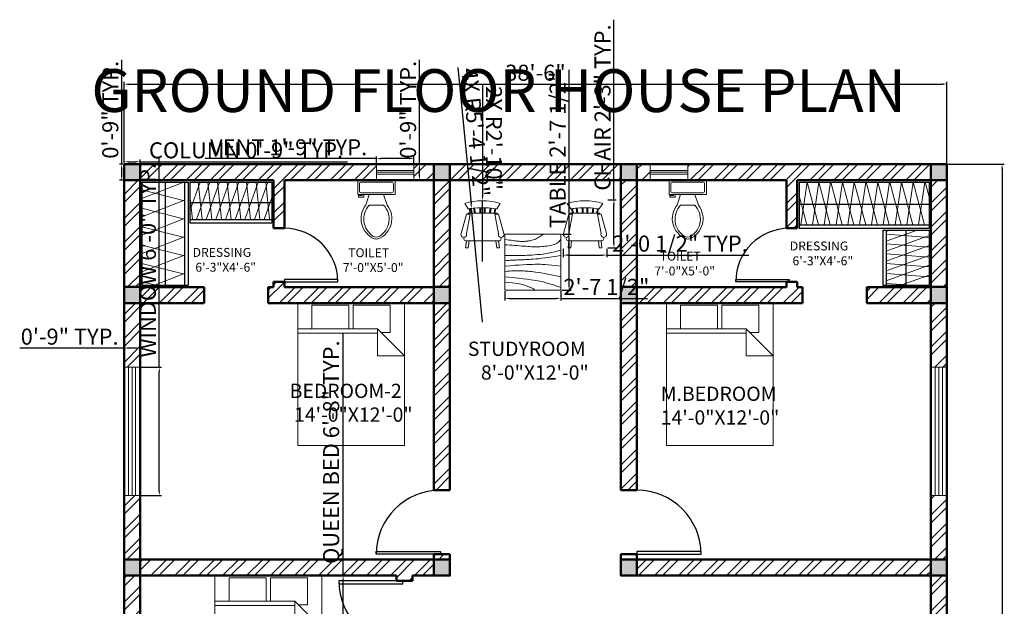
# Model space of a CAD drawing. Units: inches. Extents: x 381 to 1001, y 3003 to 3971.
# Tile 4 of 4: x 419 to 972, y 3641 to 3971. Entities that reach past the tile are written whole.
import ezdxf

# ---------------------------------------------------------------- set-up
doc = ezdxf.new("R2010")
doc.units = ezdxf.units.IN
for name, color, linetype, lineweight in [('A-ANNO-DIMS', 2, 'Continuous', 18), ('A-ANNO-TEXT', 7, 'Continuous', 25), ('A-AREA-IDEN', 7, 'Continuous', 18), ('A-COLS', 7, 'Continuous', 50), ('A-DOOR', 4, 'Continuous', 25), ('A-FLOR-CASE', 8, 'Continuous', 25), ('A-FLOR-CASE-PATT', 252, 'Continuous', 13), ('A-FLOR-FIXT', 9, 'Continuous', 18), ('A-FURN', 8, 'Continuous', 18), ('A-GLAZ', 244, 'Continuous', 18), ('A-WALL', 7, 'Continuous', 50), ('A-WALL-PATT', 252, 'Continuous', 13)]:
    doc.layers.add(name, color=color, linetype=linetype, lineweight=lineweight)
doc.styles.get("Standard").update_dxf_attribs({"font": 'arial.ttf'})
doc.dimstyles.new('ISO-25', dxfattribs={"dimtxt": 9, "dimasz": 2.5, "dimexe": 1.25, "dimexo": 0.625, "dimtad": 1, "dimlunit": 3, "dimtxsty": 'Standard', "dimcen": 2.5, "dimadec": 0, "dimazin": 0, "dimtfac": 1, "dimtmove": 0, "dimatfit": 3, "dimfxl": 1, "dimarcsym": 0})

# ---------------------------------------------------------------- blocks, each defined once
blk = doc.blocks.new('*U5')
for p, q in [((0, 0), (0, 6)), ((40, 0), (40, 6))]:
    blk.add_line(p, q)
blk.add_lwpolyline([(0, 0), (0, -40), (1.75, -40), (1.75, 0)], close=True)
blk.add_arc((0, 0), 40, 270, 360)
blk = doc.blocks.new('*U4')
for p, q in [((0, 0), (0, -6)), ((40, 0), (40, -6))]:
    blk.add_line(p, q)
blk.add_lwpolyline([(0, 0), (0, 40), (1.75, 40), (1.75, 0)], close=True)
blk.add_arc((0, 0), 40, 0, 90)
blk = doc.blocks.new('*U3')
for p, q in [((0, 0), (0, -6)), ((-40, 0), (-40, -6))]:
    blk.add_line(p, q)
blk.add_lwpolyline([(0, 0), (0, 40), (-1.75, 40), (-1.75, 0)], close=True)
blk.add_arc((0, 0), 40, 90, 180)
blk = doc.blocks.new('*U9')
for p, q in [((9.5, -6), (9.5, -2)), ((-10, -8.5), (-8, -8.5)), ((-10, -9.5), (-10, -8.5)), ((-7, -9.5), (-10, -9.5)), ((-8, -8.5), (-8, -8)), ((-7, -8), (-7, -9.5)), ((-4, -8), (-6, -14)), ((4, -8), (6, -14)), ((4, -14), (-4, -14))]:
    blk.add_line(p, q)
blk.add_lwpolyline([(10.5, -8), (10.5, 0), (-10.5, 0), (-10.5, -8)], close=True)
for points in [[(-9.5, -2), (-9.5, -6)], [(8.5, -1), (-8.5, -1)], [(-8.5, -7), (8.5, -7)]]:
    blk.add_lwpolyline(points)
for centre, radius, start, end in [((-8.62, -1.88), 0.884, 81.8699, 188.1301), ((8.62, -1.88), 0.884, 351.8699, 98.1301), ((-8.62, -6.12), 0.884, 171.8699, 278.1301), ((8.62, -6.12), 0.884, 261.8699, 8.1301), ((3.52, -21.58), 12.17, 141.4691, 247.9714), ((4.2, -21.82), 11.33, 136.3677, 238.9468), ((-3.52, -21.58), 12.17, 292.0284, 38.5307), ((-4.2, -21.82), 11.33, 301.053, 43.6321), ((0, -27.88), 4, 245.7318, 294.2682), ((0, -29), 4, 254.8605, 285.1395)]:
    blk.add_arc(centre, radius, start, end)
blk = doc.blocks.new('Bed - Queen')
for p, q in [((0, -80.00003), (0, 0)), ((0, 0), (59.99999, 0)), ((59.99999, 0), (59.99999, -80.00003)), ((7.99999, -1.2), (28.79998, -1.2)), ((7.99999, -14.4), (7.99999, -1.2)), ((28.79998, -1.2), (28.79998, -14.4)), ((31.19999, -1.2), (51.99999, -1.2)), ((31.19999, -14.4), (31.19999, -1.2)), ((51.99999, -1.2), (51.99999, -16.4)), ((0, -14.4), (44.8, -14.4)), ((59.99999, -29.6), (44.8, -14.4)), ((44.8, -14.4), (44.8, -29.6)), ((51.99999, -16.4), (46.79936, -16.4)), ((44.8, -16.8), (0, -16.8)), ((44.8, -29.6), (59.99999, -29.6)), ((59.99999, -80.00003), (0, -80.00003))]:
    blk.add_line(p, q)
blk = doc.blocks.new('Chair - Rocking')
for p, q in [((-8, -4.5), (-10, -1.5)), ((-7.5, -4.5), (-7, -7)), ((-6.5, -7), (-7.02225, -4.43)), ((-4.5, -7), (-4.96674, -4.19951)), ((-4, -7), (-4.40532, -4.16272)), ((-1.5, -4.05012), (-1.5, -7)), ((-1, -7), (-1, -4.05012)), ((1, -7), (1, -4.04655)), ((1.5, -4.05012), (1.5, -7)), ((4, -7), (4.40187, -4.18694)), ((4.5, -7), (4.96761, -4.19437)), ((6.5, -7), (7, -4.4057)), ((7.5, -4.5), (7, -7)), ((8, -4.5), (10, -1.5)), ((-9, -7.5), (-12, -18.49999)), ((-7, -7.5), (-9, -7.5)), ((-9, -18.49999), (-7, -7.5)), ((-8.23428, -6.99939), (-8.3093, -7.47958)), ((-8.23041, -7), (8.23915, -7)), ((7, -7.5), (9, -7.5)), ((9, -18.49999), (7, -7.5)), ((8.31071, -7.48854), (8.23449, -7.00073)), ((9, -7.5), (12, -18.49999)), ((-10.36644, -20.64523), (-10.5, -21.49999)), ((10.5, -21.49999), (10.3575, -20.58798)), ((-9, -22.49999), (-9.5, -26.49999)), ((0, -22.49999), (-9.5, -22.49999)), ((-9.5, -26.49999), (-8, -26.49999)), ((-8, -26.49999), (-7.5, -22.49999)), ((0, -22.49999), (9.5, -22.49999)), ((8, -26.49999), (7.5, -22.49999)), ((9.5, -26.49999), (8, -26.49999)), ((9, -22.49999), (9.5, -26.49999))]:
    blk.add_line(p, q)
for centre, radius, start, end in [((0, -34.08333), 34.08333, 72.93847, 107.0615), ((0, -68.25004), 64.25, 93.92211, 97.15267), ((0, -68.25004), 64.25, 82.84733, 93.92211), ((-10.5, -18.99999), 1.58114, 161.5651, 18.43495), ((-9.5, -21.49999), 1, 180, 270), ((10.5, -18.99999), 1.58114, 161.5651, 18.43495), ((9.5, -21.49999), 1, 270, 0)]:
    blk.add_arc(centre, radius, start, end)
blk = doc.blocks.new('Table - Square Woodgrain 42 x 42 in.')
blk.add_line((0, -42), (42, -42))
for points in [[(0, -4), (1.704, -4.2172), (3.2358, -4.4188), (4.615, -4.604), (5.8615, -4.7721), (6.9951, -4.9224), (8.0357, -5.0541), (9.0031, -5.1667), (9.9171, -5.2594), (10.7951, -5.3316), (11.6445, -5.3836), (12.4702, -5.4157), (13.277, -5.4283), (14.0698, -5.4217), (14.8535, -5.3964), (15.6331, -5.3526), (16.4133, -5.2908), (17.1986, -5.2103), (17.9913, -5.1062), (18.793, -4.9727), (19.6056, -4.8038), (20.4307, -4.5937), (21.2701, -4.3365), (22.1256, -4.0262), (22.9989, -3.6571), (23.888, -3.2272), (24.7756, -2.7516), (25.6408, -2.2491), (26.4624, -1.7387), (27.2195, -1.2395), (27.891, -0.7703), (28.456, -0.3501), (28.8934, 0.002)], [(0, -42), (0, 0), (42, 0), (42, -42)], [(0, -8), (1.8203, -8.1001), (3.6741, -8.2149), (5.5411, -8.3408), (7.4011, -8.4741), (9.2339, -8.6112), (11.0193, -8.7484), (12.7371, -8.8821), (14.3671, -9.0086), (15.8954, -9.1246), (17.3337, -9.2278), (18.6997, -9.3159), (20.0116, -9.387), (21.2871, -9.4389), (22.5442, -9.4696), (23.8008, -9.477), (25.0749, -9.459), (26.3791, -9.4137), (27.7049, -9.3403), (29.0383, -9.2382), (30.3655, -9.1068), (31.6728, -8.9455), (32.9461, -8.7535), (34.1717, -8.5304), (35.3358, -8.2756), (36.4268, -7.9863), (37.443, -7.6521), (38.3849, -7.2603), (39.253, -6.7986), (40.048, -6.2542), (40.7705, -5.6147), (41.421, -4.8674), (42, -4)], [(42, -12), (39.1784, -12.8621), (36.4519, -13.5654), (33.8246, -14.1294), (31.3004, -14.5731), (28.8832, -14.9161), (26.577, -15.1775), (24.3858, -15.3768), (22.3136, -15.5332), (20.3622, -15.6632), (18.5254, -15.7718), (16.7947, -15.8612), (15.1618, -15.9338), (13.6183, -15.9916), (12.1558, -16.0369), (10.7659, -16.0718), (9.4403, -16.0987), (8.1703, -16.1191), (6.9461, -16.1325), (5.7577, -16.1377), (4.595, -16.1335), (3.4479, -16.1188), (2.3064, -16.0924), (1.1604, -16.0532), (0, -16)], [(42, -16), (37.6529, -16.7365), (33.8802, -17.329), (30.6179, -17.7961), (27.8015, -18.1561), (25.3668, -18.4275), (23.2497, -18.6288), (21.3859, -18.7785), (19.7111, -18.8949), (18.1693, -18.9939), (16.7375, -19.0795), (15.401, -19.1534), (14.1449, -19.217), (12.9544, -19.2717), (11.8148, -19.3191), (10.7113, -19.3606), (9.6291, -19.3976), (8.5534, -19.4323), (7.47, -19.4689), (6.3643, -19.5122), (5.222, -19.5672), (4.0288, -19.6386), (2.7703, -19.7313), (1.4321, -19.8501), (0, -20)], [(0, -24), (3.9243, -23.6805), (7.4766, -23.4138), (10.6891, -23.1954), (13.5943, -23.0205), (16.2247, -22.8847), (18.6125, -22.7832), (20.7903, -22.7116), (22.7903, -22.6651), (24.6563, -22.642), (26.4764, -22.6507), (28.35, -22.7024), (30.3766, -22.8084), (32.6555, -22.98), (35.2861, -23.2283), (38.3678, -23.5645), (42, -24)], [(42, -32), (37.392, -31.017), (33.4585, -30.2231), (30.1291, -29.5949), (27.3334, -29.109), (25.0009, -28.742), (23.0612, -28.4707), (21.4439, -28.2716), (20.0786, -28.1215), (18.8998, -28.0002), (17.8609, -27.9014), (16.9206, -27.8219), (16.0371, -27.7588), (15.1691, -27.709), (14.2748, -27.6693), (13.3128, -27.6368), (12.2415, -27.6083), (11.0295, -27.5824), (9.6867, -27.5643), (8.233, -27.5608), (6.6884, -27.5787), (5.0728, -27.6248), (3.4062, -27.7058), (1.7086, -27.8286), (0, -28)], [(0, -32), (5.4026, -32.5358), (9.9494, -33.019), (13.7424, -33.4553), (16.8834, -33.8505), (19.4743, -34.2106), (21.6171, -34.5413), (23.4136, -34.8486), (24.9657, -35.1382), (26.3614, -35.4156), (27.6332, -35.6841), (28.7995, -35.9467), (29.8788, -36.2064), (30.8897, -36.4661), (31.8507, -36.7288), (32.7802, -36.9973), (33.6968, -37.2747), (34.6175, -37.5635), (35.5531, -37.8651), (36.5128, -38.1805), (37.506, -38.5108), (38.5421, -38.8568), (39.6302, -39.2197), (40.7797, -39.6004), (42, -40)], [(0, -36), (3.0098, -36.2857), (5.5354, -36.5643), (7.6368, -36.8359), (9.374, -37.1009), (10.807, -37.3597), (11.9957, -37.6126), (13.0002, -37.8599), (13.8804, -38.102), (14.6874, -38.3393), (15.4365, -38.5729), (16.1338, -38.8041), (16.7858, -39.0341), (17.3987, -39.264), (17.9787, -39.4952), (18.5322, -39.7288), (19.0655, -39.9662), (19.5832, -40.2081), (20.0842, -40.4544), (20.5657, -40.7046), (21.0249, -40.9581), (21.459, -41.2144), (21.8653, -41.4731), (22.2409, -41.7335), (22.5831, -41.9951)]]:
    blk.add_lwpolyline(points)
blk = doc.blocks.new('*D22')
at = {"layer": 'A-ANNO-DIMS', "color": 0, "lineweight": -2, "transparency": 16777216}
for p, q in [((940.7, 3889.64), (972.35, 3889.64)), ((971.1, 3887.14), (971.1, 3133.06)), ((940.7, 3130.56), (972.35, 3130.56))]:
    blk.add_line(p, q, dxfattribs=at)
at = {"layer": 'A-ANNO-DIMS', "color": 0, "transparency": 16777216}
for points in [[(970.69, 3887.14), (971.52, 3887.14), (971.1, 3889.64)], [(970.69, 3133.06), (971.52, 3133.06), (971.1, 3130.56)]]:
    blk.add_solid(points, dxfattribs=at)
at = {"layer": 'Defpoints', "color": 0, "transparency": 16777216}
for p in [(940.08, 3889.64), (940.08, 3130.56), (971.1, 3130.56)]:
    blk.add_point(p, dxfattribs=at)
at = {"layer": 'A-ANNO-DIMS', "color": 0, "transparency": 16777216, "insert": (965.88, 3510.1), "char_height": 9, "attachment_point": 5, "rotation": 90}
blk.add_mtext('63\'-3.07"', dxfattribs=at)
blk = doc.blocks.new('WIN-72X9')
for p, q in [((72, 6.5), (0, 6.5)), ((72, 4.5), (0, 4.5)), ((72, 2.5), (0, 2.5))]:
    blk.add_line(p, q)
blk.add_lwpolyline([(72, 9), (72, 0), (0, 0), (0, 9)], close=True)
blk = doc.blocks.new('VENT-WIN-21X9')
for p, q in [((3.5, 0), (3.5, 21)), ((4.5, 0), (4.5, 21)), ((5.5, 0), (5.5, 21))]:
    blk.add_line(p, q)
blk.add_lwpolyline([(9, 21), (9, 0), (0, 0), (0, 21)], close=True)
blk = doc.blocks.new('COLUMN-9X9')
h = blk.add_hatch(color=256)
h.dxf.hatch_style = 1
h.paths.add_polyline_path([(9, 9), (0, 9), (0, 0), (9, 0)])
blk.add_lwpolyline([(0, 9), (9, 9), (9, 0), (0, 0)], close=True)
blk = doc.blocks.new('*D30')
at = {"layer": 'A-ANNO-DIMS', "color": 0, "lineweight": -2, "transparency": 16777216}
for p, q in [((478.08, 3890.19), (478.08, 3892.16)), ((480.58, 3890.91), (484.58, 3890.91)), ((487.08, 3890.19), (487.08, 3892.16)), ((487.08, 3890.91), (603.56, 3890.91))]:
    blk.add_line(p, q, dxfattribs=at)
at = {"layer": 'A-ANNO-DIMS', "color": 0, "transparency": 16777216}
for points in [[(480.58, 3891.33), (480.58, 3890.5), (478.08, 3890.91)], [(484.58, 3891.33), (484.58, 3890.5), (487.08, 3890.91)]]:
    blk.add_solid(points, dxfattribs=at)
at = {"layer": 'Defpoints', "color": 0, "transparency": 16777216}
for p in [(478.08, 3889.56), (487.08, 3890.91), (487.08, 3889.56)]:
    blk.add_point(p, dxfattribs=at)
at = {"layer": 'A-ANNO-DIMS', "color": 0, "transparency": 16777216, "insert": (546.57, 3896.2), "char_height": 9, "attachment_point": 5}
blk.add_mtext('COLUMN 0\'-9" TYP.', dxfattribs=at)
blk = doc.blocks.new('*D31')
at = {"layer": 'A-ANNO-DIMS', "color": 0, "lineweight": -2, "transparency": 16777216}
for p, q in [((476.73, 3889.56), (476.73, 3948.17)), ((477.45, 3889.56), (475.48, 3889.56)), ((476.73, 3883.06), (476.73, 3887.06)), ((477.45, 3880.56), (475.48, 3880.56))]:
    blk.add_line(p, q, dxfattribs=at)
at = {"layer": 'A-ANNO-DIMS', "color": 0, "transparency": 16777216}
for points in [[(476.31, 3887.06), (477.14, 3887.06), (476.73, 3889.56)], [(476.31, 3883.06), (477.14, 3883.06), (476.73, 3880.56)]]:
    blk.add_solid(points, dxfattribs=at)
at = {"layer": 'Defpoints', "color": 0, "transparency": 16777216}
for p in [(476.73, 3889.56), (478.08, 3889.56), (478.08, 3880.56)]:
    blk.add_point(p, dxfattribs=at)
at = {"layer": 'A-ANNO-DIMS', "color": 0, "transparency": 16777216, "insert": (471.51, 3920.12), "char_height": 9, "attachment_point": 5, "rotation": 90}
blk.add_mtext('0\'-9" TYP.', dxfattribs=at)
blk = doc.blocks.new('*D32')
at = {"layer": 'A-ANNO-DIMS', "color": 0, "lineweight": -2, "transparency": 16777216}
for p, q in [((497.88, 3775.56), (497.88, 3893.2)), ((487.7, 3775.56), (499.13, 3775.56)), ((497.88, 3706.06), (497.88, 3773.06)), ((487.7, 3703.56), (499.13, 3703.56))]:
    blk.add_line(p, q, dxfattribs=at)
at = {"layer": 'A-ANNO-DIMS', "color": 0, "transparency": 16777216}
for points in [[(497.46, 3773.06), (498.29, 3773.06), (497.88, 3775.56)], [(497.46, 3706.06), (498.29, 3706.06), (497.88, 3703.56)]]:
    blk.add_solid(points, dxfattribs=at)
at = {"layer": 'Defpoints', "color": 0, "transparency": 16777216}
for p in [(487.08, 3775.56), (497.88, 3775.56), (487.08, 3703.56)]:
    blk.add_point(p, dxfattribs=at)
at = {"layer": 'A-ANNO-DIMS', "color": 0, "transparency": 16777216, "insert": (492.6, 3835.63), "char_height": 9, "attachment_point": 5, "rotation": 90}
blk.add_mtext('WINDOW 6\'-0" TYP.', dxfattribs=at)
blk = doc.blocks.new('*D33')
at = {"layer": 'A-ANNO-DIMS', "color": 0, "lineweight": -2, "transparency": 16777216}
for p, q in [((478.08, 3776.19), (478.08, 3787.61)), ((487.08, 3776.19), (487.08, 3787.61)), ((478.08, 3786.36), (419.47, 3786.36)), ((484.58, 3786.36), (480.58, 3786.36))]:
    blk.add_line(p, q, dxfattribs=at)
at = {"layer": 'A-ANNO-DIMS', "color": 0, "transparency": 16777216}
for points in [[(480.58, 3786.78), (480.58, 3785.95), (478.08, 3786.36)], [(484.58, 3786.78), (484.58, 3785.95), (487.08, 3786.36)]]:
    blk.add_solid(points, dxfattribs=at)
at = {"layer": 'Defpoints', "color": 0, "transparency": 16777216}
for p in [(478.08, 3786.36), (478.08, 3775.56), (487.08, 3775.56)]:
    blk.add_point(p, dxfattribs=at)
at = {"layer": 'A-ANNO-DIMS', "color": 0, "transparency": 16777216, "insert": (447.52, 3791.59), "char_height": 9, "attachment_point": 5}
blk.add_mtext('0\'-9" TYP.', dxfattribs=at)
blk = doc.blocks.new('*D34')
at = {"layer": 'A-ANNO-DIMS', "color": 0, "lineweight": -2, "transparency": 16777216}
for p, q in [((619.78, 3892.71), (523.68, 3892.71)), ((619.78, 3890.19), (619.78, 3893.96)), ((638.28, 3892.71), (622.28, 3892.71)), ((640.78, 3890.19), (640.78, 3893.96))]:
    blk.add_line(p, q, dxfattribs=at)
at = {"layer": 'A-ANNO-DIMS', "color": 0, "transparency": 16777216}
for points in [[(622.28, 3893.13), (622.28, 3892.3), (619.78, 3892.71)], [(638.28, 3893.13), (638.28, 3892.3), (640.78, 3892.71)]]:
    blk.add_solid(points, dxfattribs=at)
at = {"layer": 'Defpoints', "color": 0, "transparency": 16777216}
for p in [(619.78, 3892.71), (619.78, 3889.56), (640.78, 3889.56)]:
    blk.add_point(p, dxfattribs=at)
at = {"layer": 'A-ANNO-DIMS', "color": 0, "transparency": 16777216, "insert": (570.48, 3897.94), "char_height": 9, "attachment_point": 5}
blk.add_mtext('VENT 1\'-9" TYP.', dxfattribs=at)
blk = doc.blocks.new('*D35')
at = {"layer": 'A-ANNO-DIMS', "color": 0, "lineweight": -2, "transparency": 16777216}
for p, q in [((643.93, 3889.56), (643.93, 3948.17)), ((641.41, 3889.56), (645.18, 3889.56)), ((643.93, 3883.06), (643.93, 3887.06)), ((641.41, 3880.56), (645.18, 3880.56))]:
    blk.add_line(p, q, dxfattribs=at)
at = {"layer": 'A-ANNO-DIMS', "color": 0, "transparency": 16777216}
for points in [[(643.51, 3887.06), (644.35, 3887.06), (643.93, 3889.56)], [(643.51, 3883.06), (644.35, 3883.06), (643.93, 3880.56)]]:
    blk.add_solid(points, dxfattribs=at)
at = {"layer": 'Defpoints', "color": 0, "transparency": 16777216}
for p in [(640.78, 3889.56), (643.93, 3889.56), (640.78, 3880.56)]:
    blk.add_point(p, dxfattribs=at)
at = {"layer": 'A-ANNO-DIMS', "color": 0, "transparency": 16777216, "insert": (638.71, 3920.12), "char_height": 9, "attachment_point": 5, "rotation": 90}
blk.add_mtext('0\'-9" TYP.', dxfattribs=at)
blk = doc.blocks.new('*D36')
at = {"layer": 'A-ANNO-DIMS', "color": 0, "lineweight": -2, "transparency": 16777216}
for p, q in [((601.08, 3658.56), (601.08, 3794.71)), ((589.7, 3658.56), (602.33, 3658.56)), ((601.08, 3581.06), (601.08, 3656.06)), ((589.7, 3578.56), (602.33, 3578.56))]:
    blk.add_line(p, q, dxfattribs=at)
at = {"layer": 'A-ANNO-DIMS', "color": 0, "transparency": 16777216}
for points in [[(600.66, 3656.06), (601.49, 3656.06), (601.08, 3658.56)], [(600.66, 3581.06), (601.49, 3581.06), (601.08, 3578.56)]]:
    blk.add_solid(points, dxfattribs=at)
at = {"layer": 'Defpoints', "color": 0, "transparency": 16777216}
for p in [(589.08, 3658.56), (601.08, 3658.56), (589.08, 3578.56)]:
    blk.add_point(p, dxfattribs=at)
at = {"layer": 'A-ANNO-DIMS', "color": 0, "transparency": 16777216, "insert": (595.52, 3727.89), "char_height": 9, "attachment_point": 5, "rotation": 90}
blk.add_mtext('QUEEN BED 6\'-8" TYP.', dxfattribs=at)
blk = doc.blocks.new('*D40')
at = {"layer": 'A-ANNO-DIMS', "color": 0, "lineweight": -2, "transparency": 16777216}
for p, q in [((753.17, 3869.59), (753.17, 3970.7)), ((749.74, 3869.59), (754.42, 3869.59)), ((753.17, 3845.09), (753.17, 3867.09)), ((749.74, 3842.59), (754.42, 3842.59))]:
    blk.add_line(p, q, dxfattribs=at)
at = {"layer": 'A-ANNO-DIMS', "color": 0, "transparency": 16777216}
for points in [[(752.75, 3867.09), (753.58, 3867.09), (753.17, 3869.59)], [(752.75, 3845.09), (753.58, 3845.09), (753.17, 3842.59)]]:
    blk.add_solid(points, dxfattribs=at)
at = {"layer": 'Defpoints', "color": 0, "transparency": 16777216}
for p in [(749.12, 3869.59), (753.17, 3869.59), (749.12, 3842.59)]:
    blk.add_point(p, dxfattribs=at)
at = {"layer": 'A-ANNO-DIMS', "color": 0, "transparency": 16777216, "insert": (747.89, 3921.4), "char_height": 9, "attachment_point": 5, "rotation": 90}
blk.add_mtext('CHAIR 2\'-3" TYP.', dxfattribs=at)
blk = doc.blocks.new('*D41')
at = {"layer": 'A-ANNO-DIMS', "color": 0, "lineweight": -2, "transparency": 16777216}
for p, q in [((724.68, 3841.96), (724.68, 3837.29)), ((727.18, 3838.54), (746.62, 3838.54)), ((749.12, 3841.96), (749.12, 3837.29)), ((749.12, 3838.54), (828.85, 3838.54))]:
    blk.add_line(p, q, dxfattribs=at)
at = {"layer": 'A-ANNO-DIMS', "color": 0, "transparency": 16777216}
for points in [[(727.18, 3838.95), (727.18, 3838.12), (724.68, 3838.54)], [(746.62, 3838.95), (746.62, 3838.12), (749.12, 3838.54)]]:
    blk.add_solid(points, dxfattribs=at)
at = {"layer": 'Defpoints', "color": 0, "transparency": 16777216}
for p in [(724.68, 3842.59), (749.12, 3842.59), (749.12, 3838.54)]:
    blk.add_point(p, dxfattribs=at)
at = {"layer": 'A-ANNO-DIMS', "color": 0, "transparency": 16777216, "insert": (790.24, 3843.82), "char_height": 9, "attachment_point": 5}
blk.add_mtext('2\'-0 1/2" TYP.', dxfattribs=at)
blk = doc.blocks.new('*D52')
at = {"layer": 'A-ANNO-DIMS', "color": 0, "lineweight": -2, "transparency": 16777216}
for p, q in [((727.96, 3850.27), (727.96, 3942.47)), ((723.88, 3850.27), (729.21, 3850.27)), ((727.96, 3821.42), (727.96, 3847.77)), ((723.88, 3818.92), (729.21, 3818.92))]:
    blk.add_line(p, q, dxfattribs=at)
at = {"layer": 'A-ANNO-DIMS', "color": 0, "transparency": 16777216}
for points in [[(727.54, 3847.77), (728.38, 3847.77), (727.96, 3850.27)], [(727.54, 3821.42), (728.38, 3821.42), (727.96, 3818.92)]]:
    blk.add_solid(points, dxfattribs=at)
at = {"layer": 'Defpoints', "color": 0, "transparency": 16777216}
for p in [(723.26, 3850.27), (727.96, 3850.27), (723.26, 3818.92)]:
    blk.add_point(p, dxfattribs=at)
at = {"layer": 'A-ANNO-DIMS', "color": 0, "transparency": 16777216, "insert": (722.68, 3897.62), "char_height": 9, "attachment_point": 5, "rotation": 90}
blk.add_mtext('TABLE 2\'-7 1/2"', dxfattribs=at)
blk = doc.blocks.new('*D53')
at = {"layer": 'A-ANNO-DIMS', "color": 0, "lineweight": -2, "transparency": 16777216}
for p, q in [((691.91, 3818.3), (691.91, 3812.97)), ((723.26, 3818.3), (723.26, 3812.97)), ((694.41, 3814.22), (720.76, 3814.22)), ((723.26, 3814.22), (772.06, 3814.22))]:
    blk.add_line(p, q, dxfattribs=at)
at = {"layer": 'A-ANNO-DIMS', "color": 0, "transparency": 16777216}
for points in [[(694.41, 3814.64), (694.41, 3813.8), (691.91, 3814.22)], [(720.76, 3814.64), (720.76, 3813.8), (723.26, 3814.22)]]:
    blk.add_solid(points, dxfattribs=at)
at = {"layer": 'Defpoints', "color": 0, "transparency": 16777216}
for p in [(691.91, 3818.92), (723.26, 3818.92), (723.26, 3814.22)]:
    blk.add_point(p, dxfattribs=at)
at = {"layer": 'A-ANNO-DIMS', "color": 0, "transparency": 16777216, "insert": (748.91, 3819.5), "char_height": 9, "attachment_point": 5}
blk.add_mtext('2\'-7 1/2"', dxfattribs=at)
blk = doc.blocks.new('*D54')
at = {"layer": 'A-ANNO-DIMS', "color": 0, "lineweight": -2, "transparency": 16777216}
for p, q in [((478.08, 3890.19), (478.07, 3935.76)), ((480.57, 3934.52), (937.57, 3934.59)), ((940.08, 3890.26), (940.07, 3935.84))]:
    blk.add_line(p, q, dxfattribs=at)
at = {"layer": 'A-ANNO-DIMS', "color": 0, "transparency": 16777216}
for points in [[(480.57, 3934.93), (480.57, 3934.1), (478.07, 3934.51)], [(937.57, 3935), (937.57, 3934.17), (940.07, 3934.59)]]:
    blk.add_solid(points, dxfattribs=at)
at = {"layer": 'Defpoints', "color": 0, "transparency": 16777216}
for p in [(940.07, 3934.59), (478.08, 3889.56), (940.08, 3889.64)]:
    blk.add_point(p, dxfattribs=at)
at = {"layer": 'A-ANNO-DIMS', "color": 0, "transparency": 16777216, "insert": (709.07, 3939.77), "char_height": 9, "attachment_point": 5, "rotation": 0.0089}
blk.add_mtext('38\'-6"', dxfattribs=at)
blk = doc.blocks.new('*D63')
at = {"layer": 'A-ANNO-DIMS', "color": 0, "lineweight": -2, "transparency": 16777216}
for p, q in [((665.47, 3943.88), (672.9, 3867.28)), ((679.34, 3800.84), (673.14, 3864.79))]:
    blk.add_line(p, q, dxfattribs=at)
at = {"layer": 'A-ANNO-DIMS', "color": 0, "transparency": 16777216}
blk.add_solid([(673.31, 3867.32), (672.48, 3867.24), (673.14, 3864.79)], dxfattribs=at)
at = {"layer": 'Defpoints', "color": 0, "transparency": 16777216}
for p in [(673.14, 3864.79), (679.34, 3800.84)]:
    blk.add_point(p, dxfattribs=at)
at = {"layer": 'A-ANNO-DIMS', "color": 0, "transparency": 16777216, "insert": (674.32, 3907.33), "char_height": 9, "attachment_point": 5, "rotation": 275.5377}
blk.add_mtext('4X R5\'-4 1/2"', dxfattribs=at)
blk = doc.blocks.new('*D64')
at = {"layer": 'A-ANNO-DIMS', "color": 0, "lineweight": -2, "transparency": 16777216}
for p, q in [((679.34, 3934.36), (679.34, 3871.59)), ((679.34, 3835), (679.34, 3869.09))]:
    blk.add_line(p, q, dxfattribs=at)
at = {"layer": 'A-ANNO-DIMS', "color": 0, "transparency": 16777216}
blk.add_solid([(679.75, 3871.59), (678.92, 3871.59), (679.34, 3869.09)], dxfattribs=at)
at = {"layer": 'Defpoints', "color": 0, "transparency": 16777216}
for p in [(679.34, 3869.09), (679.34, 3835)]:
    blk.add_point(p, dxfattribs=at)
at = {"layer": 'A-ANNO-DIMS', "color": 0, "transparency": 16777216, "insert": (684.56, 3904.22), "char_height": 9, "attachment_point": 5, "rotation": 270.0003}
blk.add_mtext('2X R2\'-10"', dxfattribs=at)

msp = doc.modelspace()

# ---------------------------------------------------------------- hatches: boundary and pattern name
at = {"layer": 'A-FLOR-CASE-PATT'}
h = msp.add_hatch(dxfattribs=at)
h.set_pattern_fill('ANSI31', color=256, scale=3.01979, angle=-23.5238, style=0)
h.paths.add_polyline_path([(488.078, 3821.565), (512.078, 3821.565), (512.078, 3879.565), (488.078, 3879.565)])
h = msp.add_hatch(dxfattribs=at)
h.set_pattern_fill('ANSI31', color=256, scale=3.147409, angle=120.9056, style=0)
h.paths.add_polyline_path([(488.078, 3821.565), (512.078, 3821.565), (512.078, 3879.565), (488.078, 3879.565)])
h = msp.add_hatch(dxfattribs=at)
h.set_pattern_fill('ANSI31', color=256, scale=1.610526, angle=25.59606, style=0)
h.paths.add_polyline_path([(515.078, 3858.565), (561.078, 3858.565), (561.078, 3879.565), (515.078, 3879.565)])
h = msp.add_hatch(dxfattribs=at)
h.set_pattern_fill('ANSI31', color=256, scale=1.698905, angle=50.75558, style=0)
h.paths.add_polyline_path([(515.078, 3858.565), (561.078, 3858.565), (561.078, 3879.565), (515.078, 3879.565)])
h = msp.add_hatch(dxfattribs=at)
h.set_pattern_fill('ANSI31', color=256, scale=2.014967, angle=59.89108, style=0)
h.paths.add_polyline_path([(857.078, 3855.565), (930.078, 3855.565), (930.078, 3879.565), (857.078, 3879.565)])
h = msp.add_hatch(dxfattribs=at)
h.set_pattern_fill('ANSI31', color=256, scale=2.06231, angle=36.5415, style=0)
h.paths.add_polyline_path([(857.078, 3855.565), (930.078, 3855.565), (930.078, 3879.565), (857.078, 3879.565)])
h = msp.add_hatch(dxfattribs=at)
h.set_pattern_fill('ANSI31', color=256, scale=1.639371, angle=-25.02035, style=0)
h.paths.add_polyline_path([(906.078, 3821.565), (930.078, 3821.565), (930.078, 3852.565), (906.078, 3852.565)])
h = msp.add_hatch(dxfattribs=at)
h.set_pattern_fill('ANSI31', color=256, scale=1.739058, angle=130.5331, style=0)
h.paths.add_polyline_path([(906.078, 3821.565), (930.078, 3821.565), (930.078, 3852.565), (906.078, 3852.565)])
at = {"layer": 'A-WALL-PATT'}
h = msp.add_hatch(dxfattribs=at)
h.set_pattern_fill('ANSI32', color=256)
h.paths.add_polyline_path([(652.078, 3667.565), (487.078, 3667.565), (487.078, 3658.565), (631.078, 3658.565), (631.078, 3655.565), (634.678, 3655.565), (640.078, 3655.565), (640.078, 3658.565), (652.078, 3658.565)])
h.paths.add_polyline_path([(487.078, 3658.637), (478.078, 3658.637), (478.078, 3634.565), (487.078, 3634.565)])
h.paths.add_polyline_path([(487.078, 3703.565), (478.078, 3703.565), (478.078, 3667.637), (487.078, 3667.637)])
h.paths.add_polyline_path([(661.078, 3811.637), (652.078, 3811.637), (652.078, 3706.565), (661.078, 3706.565)])
h.paths.add_polyline_path([(661.078, 3670.565), (655.678, 3670.565), (652.078, 3670.565), (652.078, 3667.637), (661.078, 3667.637)])
h.paths.add_polyline_path([(487.078, 3811.637), (478.078, 3811.637), (478.078, 3775.565), (487.078, 3775.565)])
h.paths.add_polyline_path([(487.078, 3880.565), (478.078, 3880.565), (478.078, 3820.637), (487.078, 3820.637)])
h.paths.add_polyline_path([(661.078, 3880.637), (652.078, 3880.637), (652.078, 3820.637), (661.078, 3820.637)])
h.paths.add_polyline_path([(652.078, 3820.565), (568.078, 3820.565), (568.078, 3823.565), (563.578, 3823.565), (562.078, 3823.565), (562.078, 3820.565), (559.078, 3820.565), (559.078, 3811.565), (652.078, 3811.565), (652.078, 3811.637)])
h.paths.add_polyline_path([(523.078, 3820.565), (487.078, 3820.565), (487.078, 3811.565), (523.078, 3811.565)])
h.paths.add_polyline_path([(619.798, 3889.565), (487.078, 3889.565), (487.078, 3880.565), (562.078, 3880.565), (562.078, 3853.565), (568.078, 3853.565), (568.078, 3880.565), (619.798, 3880.565)])
h.paths.add_polyline_path([(652.078, 3889.565), (640.798, 3889.565), (640.798, 3880.565), (652.078, 3880.565), (652.078, 3880.637)])
h.paths.add_polyline_path([(757.078, 3889.565), (661.078, 3889.565), (661.078, 3880.565), (757.078, 3880.565)])
h.paths.add_polyline_path([(766.078, 3880.637), (757.078, 3880.637), (757.078, 3820.637), (766.078, 3820.637)])
h.paths.add_polyline_path([(773.578, 3889.565), (766.078, 3889.565), (766.078, 3880.565), (773.578, 3880.565)])
h.paths.add_polyline_path([(931.078, 3889.565), (794.578, 3889.565), (794.578, 3880.565), (850.078, 3880.565), (850.078, 3853.565), (856.078, 3853.565), (856.078, 3880.565), (931.078, 3880.565)])
h.paths.add_polyline_path([(859.078, 3820.565), (856.078, 3820.565), (856.078, 3823.565), (850.078, 3823.565), (850.078, 3820.565), (766.078, 3820.565), (766.078, 3811.565), (859.078, 3811.565)])
h.paths.add_polyline_path([(940.078, 3880.637), (931.078, 3880.637), (931.078, 3820.637), (940.078, 3820.637)])
h.paths.add_polyline_path([(931.078, 3820.565), (895.078, 3820.565), (895.078, 3811.565), (931.078, 3811.565)])
h.paths.add_polyline_path([(940.078, 3811.637), (931.078, 3811.637), (931.078, 3775.565), (940.078, 3775.565)])
h.paths.add_polyline_path([(766.078, 3811.637), (757.078, 3811.637), (757.078, 3706.565), (766.078, 3706.565)])
h.paths.add_polyline_path([(940.078, 3703.565), (931.078, 3703.565), (931.078, 3667.637), (940.078, 3667.637)])
h.paths.add_polyline_path([(931.078, 3667.565), (766.078, 3667.565), (766.078, 3658.565), (931.078, 3658.565)])
h.paths.add_polyline_path([(940.078, 3658.637), (931.078, 3658.637), (931.078, 3621.065), (940.078, 3621.065)])
h.paths.add_polyline_path([(940.078, 3549.065), (931.078, 3549.065), (931.078, 3511.637), (940.078, 3511.637)])
h.paths.add_polyline_path([(931.078, 3511.565), (847.078, 3511.565), (847.078, 3502.565), (931.078, 3502.565)])
h.paths.add_polyline_path([(802.078, 3511.565), (712.078, 3511.565), (712.078, 3502.565), (802.078, 3502.565)])
h.paths.add_polyline_path([(712.078, 3502.637), (703.078, 3502.637), (703.078, 3355.637), (712.078, 3355.637)])
h.paths.add_polyline_path([(740.578, 3355.565), (712.078, 3355.565), (712.078, 3346.565), (740.578, 3346.565)])
h.paths.add_polyline_path([(841.078, 3355.565), (812.578, 3355.565), (812.578, 3346.565), (841.078, 3346.565)])
h.paths.add_polyline_path([(850.078, 3412.565), (841.078, 3412.565), (841.078, 3355.637), (850.078, 3355.637)], flags=17)
h.paths.add_polyline_path([(940.078, 3502.637), (931.078, 3502.637), (931.078, 3454.565), (841.078, 3454.565), (841.078, 3442.565), (850.078, 3442.565), (850.078, 3445.565), (931.078, 3445.565), (931.078, 3355.637), (940.078, 3355.637)])
h.paths.add_polyline_path([(931.078, 3355.565), (850.078, 3355.565), (850.078, 3346.565), (931.078, 3346.565)])
h.paths.add_polyline_path([(712.078, 3346.637), (703.078, 3346.637), (703.078, 3304.565), (700.078, 3304.565), (700.078, 3295.565), (712.078, 3295.565)])
h.paths.add_polyline_path([(622.078, 3202.565), (487.078, 3202.565), (487.078, 3193.565), (622.078, 3193.565)])
h.paths.add_polyline_path([(487.078, 3295.637), (478.078, 3295.637), (478.078, 3202.637), (487.078, 3202.637)])
h.paths.add_polyline_path([(712.078, 3295.565), (703.078, 3295.565), (703.078, 3202.565), (712.078, 3202.565)])

# ---------------------------------------------------------------- linework, layer by layer
at = {"layer": 'A-FLOR-CASE'}
for p, q in [((488.078, 3879.565), (514.078, 3879.565)), ((488.078, 3879.565), (488.078, 3821.565)), ((501.078, 3879.565), (501.078, 3821.565)), ((512.078, 3879.565), (512.078, 3821.565)), ((514.078, 3879.565), (514.078, 3821.565)), ((515.078, 3879.565), (515.078, 3856.565)), ((515.078, 3879.565), (561.078, 3879.565)), ((561.078, 3879.565), (561.078, 3856.565)), ((857.078, 3879.565), (930.078, 3879.565)), ((857.078, 3879.565), (857.078, 3853.565)), ((930.078, 3879.565), (930.078, 3853.565)), ((515.078, 3868.065), (561.078, 3868.065)), ((857.078, 3867.065), (930.078, 3867.065)), ((515.078, 3858.565), (561.078, 3858.565)), ((515.078, 3856.565), (561.078, 3856.565)), ((857.078, 3855.565), (930.078, 3855.565)), ((857.078, 3853.565), (930.078, 3853.565)), ((904.078, 3852.565), (904.078, 3821.565)), ((904.078, 3852.565), (930.078, 3852.565)), ((906.078, 3852.565), (906.078, 3821.565)), ((917.078, 3852.565), (917.078, 3821.565)), ((930.078, 3852.565), (930.078, 3821.565)), ((488.078, 3821.565), (514.078, 3821.565)), ((904.078, 3821.565), (930.078, 3821.565))]:
    msp.add_line(p, q, dxfattribs=at)
at = {"layer": 'A-WALL'}
for p, q in [((478.078, 3889.565), (478.078, 3193.565)), ((478.078, 3889.565), (940.078, 3889.565)), ((940.078, 3889.565), (940.078, 3130.565)), ((487.078, 3880.565), (562.078, 3880.565)), ((487.078, 3880.565), (487.078, 3820.565)), ((562.078, 3880.565), (562.078, 3853.565)), ((568.078, 3880.565), (568.078, 3853.565)), ((568.078, 3880.565), (652.078, 3880.565)), ((652.078, 3880.565), (652.078, 3820.565)), ((661.078, 3880.565), (661.078, 3706.565)), ((661.078, 3880.565), (757.078, 3880.565)), ((757.078, 3880.565), (757.078, 3706.565)), ((766.078, 3880.565), (766.078, 3820.565)), ((766.078, 3880.565), (850.078, 3880.565)), ((850.078, 3880.565), (850.078, 3853.565)), ((856.078, 3880.565), (856.078, 3853.565)), ((856.078, 3880.565), (931.078, 3880.565)), ((931.078, 3880.565), (931.078, 3820.565)), ((568.078, 3853.565), (562.078, 3853.565)), ((856.078, 3853.565), (850.078, 3853.565)), ((487.078, 3820.565), (523.078, 3820.565)), ((523.078, 3820.565), (523.078, 3811.565)), ((559.078, 3820.565), (559.078, 3811.565)), ((559.078, 3820.565), (562.078, 3820.565)), ((568.078, 3823.565), (562.078, 3823.565)), ((562.078, 3823.565), (562.078, 3820.565)), ((568.078, 3823.565), (568.078, 3820.565)), ((568.078, 3820.565), (652.078, 3820.565)), ((766.078, 3820.565), (850.078, 3820.565)), ((856.078, 3823.565), (850.078, 3823.565)), ((850.078, 3823.565), (850.078, 3820.565)), ((856.078, 3823.565), (856.078, 3820.565)), ((856.078, 3820.565), (859.078, 3820.565)), ((859.078, 3820.565), (859.078, 3811.565)), ((895.078, 3820.565), (895.078, 3811.565)), ((895.078, 3820.565), (931.078, 3820.565)), ((487.078, 3811.565), (523.078, 3811.565)), ((487.078, 3811.565), (487.078, 3667.565)), ((559.078, 3811.565), (652.078, 3811.565)), ((652.078, 3811.565), (652.078, 3706.565)), ((766.078, 3811.565), (859.078, 3811.565)), ((766.078, 3811.565), (766.078, 3706.565)), ((895.078, 3811.565), (931.078, 3811.565)), ((931.078, 3811.565), (931.078, 3667.565)), ((652.078, 3706.565), (661.078, 3706.565)), ((766.078, 3706.565), (757.078, 3706.565)), ((487.078, 3667.565), (652.078, 3667.565)), ((652.078, 3670.565), (661.078, 3670.565)), ((652.078, 3670.565), (652.078, 3667.565)), ((661.078, 3670.565), (661.078, 3658.565)), ((766.078, 3670.565), (757.078, 3670.565)), ((757.078, 3670.565), (757.078, 3658.565)), ((766.078, 3670.565), (766.078, 3667.565)), ((766.078, 3667.565), (931.078, 3667.565)), ((487.078, 3658.565), (631.078, 3658.565)), ((487.078, 3658.565), (487.078, 3538.565)), ((631.078, 3658.565), (631.078, 3655.565)), ((631.078, 3655.565), (640.078, 3655.565)), ((640.078, 3658.565), (640.078, 3655.565)), ((640.078, 3658.565), (661.078, 3658.565)), ((757.078, 3658.565), (931.078, 3658.565)), ((931.078, 3658.565), (931.078, 3511.565))]:
    msp.add_line(p, q, dxfattribs=at)

# ---------------------------------------------------------------- block references
at = {"layer": 'A-COLS'}
for p in [(478.078, 3880.565), (652.078, 3880.637), (757.078, 3880.637), (931.078, 3880.637), (478.078, 3811.637), (652.078, 3811.637), (757.078, 3811.637), (931.078, 3811.637), (478.078, 3658.637), (652.078, 3658.637), (757.078, 3658.637), (931.078, 3658.637)]:
    msp.add_blockref('COLUMN-9X9', p, dxfattribs=at)
at = {"layer": 'A-DOOR', "rotation": 90}
for name, p, xscale, yscale, zscale in [('*U5', (568.078, 3823.565), 0.75, 0.75, 0.75), ('*U4', (851.578, 3823.565), 0.75, 0.75, 0.75), ('*U4', (655.678, 3670.565), 0.9, 0.9, 0.9), ('*U5', (766.078, 3670.565), 0.9, 0.9, 0.9), ('*U3', (634.678, 3655.565), 0.9, 0.9, 0.9)]:
    msp.add_blockref(name, p, dxfattribs=dict(at, xscale=xscale, yscale=yscale, zscale=zscale))
at = {"layer": 'A-FLOR-FIXT'}
for p in [(619.798, 3880.565), (794.578, 3880.565)]:
    msp.add_blockref('*U9', p, dxfattribs=at)
at = {"layer": 'A-FURN'}
for name, p in [('Chair - Rocking', (679.338, 3869.088)), ('Chair - Rocking', (736.9, 3869.088)), ('Bed - Queen', (575.578, 3811.565)), ('Bed - Queen', (782.578, 3811.565)), ('Bed - Queen', (529.078, 3658.565))]:
    msp.add_blockref(name, p, dxfattribs=at)
at = {"layer": 'A-FURN', "xscale": 0.7464492223045336, "yscale": 0.7464492223045336, "zscale": 0.7464492223045336}
msp.add_blockref('Table - Square Woodgrain 42 x 42 in.', (691.905, 3850.272), dxfattribs=at)
at = {"layer": 'A-GLAZ'}
for name, p, rotation in [('VENT-WIN-21X9', (640.78, 3880.565), 89.99999999999767), ('VENT-WIN-21X9', (794.578, 3880.565), 89.99999999999785), ('WIN-72X9', (487.078, 3703.565), 90.00000000000006), ('WIN-72X9', (940.078, 3703.565), 89.99999999999996)]:
    msp.add_blockref(name, p, dxfattribs=dict(at, rotation=rotation))

# ---------------------------------------------------------------- texts
at = {"layer": 'A-ANNO-TEXT', "insert": (459.716, 3942.9), "char_height": 24, "attachment_point": 1}
msp.add_mtext_dynamic_manual_height_columns('GROUND FLOOR HOUSE PLAN', width=508.46719, gutter_width=12.5, heights=[0], dxfattribs=at)
at = {"layer": 'A-AREA-IDEN', "attachment_point": 1}
for s, width, insert, char_height in [('DRESSING\\P 6\'-3"X4\'-6"', 35.864, (516.587, 3842.554), 5), ('DRESSING\\P 6\'-3"X4\'-6"', 35.864, (851.908, 3846.155), 5), ('  TOILET\\P7\'-0"X5\'-0"', 32.42882, (600.931, 3842.373), 5), ('  TOILET\\P7\'-0"X5\'-0"', 32.42882, (775.844, 3840.451), 5), ('STUDYROOM\\P   8\'-0"X12\'-0"', 76.11512, (671.115, 3789.939), 8), ('BEDROOM-2\\P 14\'-0"X12\'-0"', 71.44563, (571.07, 3766.31), 8), ('M.BEDROOM\\P 14\'-0"X12\'-0"', 69.00419, (779.429, 3764.682), 8)]:
    msp.add_mtext_dynamic_manual_height_columns(s, width=width, gutter_width=12.5, heights=[0], dxfattribs=dict(at, insert=insert, char_height=char_height))

# ---------------------------------------------------------------- dimensions: what is measured, and where the dimension line sits
at = {"layer": 'A-ANNO-DIMS'}
for base, p1, p2, angle, text, picture, middle in [((753.168, 3869.588), (749.118, 3842.588), (749.118, 3869.588), 90, 'CHAIR <> TYP.', '*D40', (747.886, 3921.396)), ((476.728, 3889.565), (478.078, 3880.565), (478.078, 3889.565), 90, '<> TYP.', '*D31', (471.508, 3920.12)), ((643.93, 3889.565), (640.78, 3880.565), (640.78, 3889.565), 90, '<> TYP.', '*D35', (638.71, 3920.12)), ((727.959, 3850.274), (723.256, 3818.922), (723.256, 3850.274), 90, 'TABLE <>', '*D52', (722.681, 3897.622)), ((619.78, 3892.715), (640.78, 3889.565), (619.78, 3889.565), 180, 'VENT <> TYP.', '*D34', (570.48, 3897.935)), ((497.878, 3775.565), (487.078, 3703.565), (487.078, 3775.565), 90, 'WINDOW <> TYP.', '*D32', (492.597, 3835.634)), ((478.078, 3786.365), (487.078, 3775.565), (478.078, 3775.565), 180, '<> TYP.', '*D33', (447.524, 3791.585)), ((601.078, 3658.565), (589.078, 3578.565), (589.078, 3658.565), 90, 'QUEEN BED <> TYP.', '*D36', (595.524, 3727.885))]:
    dim = msp.add_linear_dim(base=base, p1=p1, p2=p2, angle=angle, text=text, dimstyle='ISO-25', override={"dimdec": 1, "dimlfac": 1, "dimrnd": 0, "dimzin": 1, "dimdsep": 46, "dimlunit": 4, "dimfrac": 2}, dxfattribs=at)
    dim.commit()
    dim.dimension.update_dxf_attribs({"geometry": picture, "text_midpoint": middle})
for base, p1, p2, angle, override, picture, middle in [((940.071, 3934.587), (478.078, 3889.565), (940.078, 3889.637), 0.00894, {"dimdec": 1, "dimlfac": 1, "dimrnd": 0, "dimzin": 1, "dimdsep": 46, "dimlunit": 4, "dimfrac": 2}, '*D54', (709.07, 3939.774)), ((971.102, 3130.565), (940.078, 3889.637), (940.078, 3130.565), 90, {"dimclrd": 0, "dimclre": 0, "dimclrt": 0}, '*D22', (965.879, 3510.101))]:
    dim = msp.add_linear_dim(base=base, p1=p1, p2=p2, angle=angle, dimstyle='ISO-25', override=override, dxfattribs=at)
    dim.commit()
    dim.dimension.update_dxf_attribs({"geometry": picture, "text_midpoint": middle})
for center, mpoint, text, picture, middle in [((679.3382, 3800.83789), (673.138, 3864.78803), '4X <>', '*D63', (674.31662, 3907.33003)), ((679.338, 3835.005), (679.338, 3869.088), '2X <>', '*D64', (684.558, 3904.224))]:
    dim = msp.add_radius_dim(center=center, mpoint=mpoint, text=text, dimstyle='ISO-25', override={"dimdec": 1, "dimlfac": 1, "dimrnd": 0, "dimzin": 1, "dimdsep": 46, "dimlunit": 4, "dimfrac": 2}, dxfattribs=at)
    dim.commit()
    dim.dimension.update_dxf_attribs({"geometry": picture, "text_midpoint": middle})
for base, p1, p2, text, picture, middle in [((487.078, 3890.915), (478.078, 3889.565), (487.078, 3889.565), 'COLUMN <> TYP.', '*D30', (546.57, 3896.196)), ((749.118, 3838.538), (724.683, 3842.588), (749.118, 3842.588), '<> TYP.', '*D41', (790.235, 3843.816))]:
    dim = msp.add_linear_dim(base=base, p1=p1, p2=p2, text=text, dimstyle='ISO-25', override={"dimdec": 1, "dimlfac": 1, "dimrnd": 0, "dimzin": 1, "dimdsep": 46, "dimlunit": 4, "dimfrac": 2}, dxfattribs=at)
    dim.commit()
    dim.dimension.update_dxf_attribs({"geometry": picture, "text_midpoint": middle})
dim = msp.add_linear_dim(base=(723.256, 3814.219), p1=(691.905, 3818.922), p2=(723.256, 3818.922), dimstyle='ISO-25', override={"dimdec": 1, "dimlfac": 1, "dimrnd": 0, "dimzin": 1, "dimdsep": 46, "dimlunit": 4, "dimfrac": 2}, dxfattribs=at)
dim.commit()
dim.dimension.update_dxf_attribs({"geometry": '*D53', "text_midpoint": (748.906, 3819.497)})

doc.saveas('drawing.dxf')
